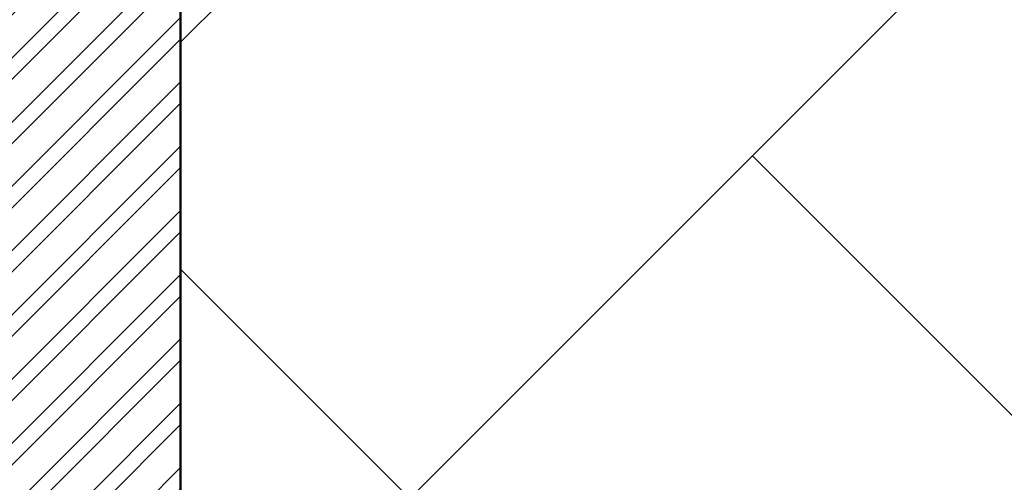
# Model space of a CAD drawing. Units: inches. Extents: x 3590 to 5167, y 65 to 1917.
# Tile 54 of 100: x 4927 to 4968, y 1538 to 1558. Entities that reach past the tile are written whole.
import ezdxf

# ---------------------------------------------------------------- set-up
doc = ezdxf.new("R2010")
doc.units = ezdxf.units.IN
for name, color, linetype, lineweight in [('A-FLOR-PATT', 8, 'Continuous', 13), ('A-WALL', 7, 'Continuous', 50), ('A-WALL-PATT', 251, 'Continuous', 13)]:
    doc.layers.add(name, color=color, linetype=linetype, lineweight=lineweight)

msp = doc.modelspace()

# ---------------------------------------------------------------- hatches: boundary and pattern name
at = {"layer": 'A-FLOR-PATT', "transparency": 33554687}
h = msp.add_hatch(dxfattribs=at)
h.set_pattern_fill('AR-HBONE', color=256, scale=0.2)
h.set_pattern_definition([(45, (-588.972, 0), (0, 28.73682), [60.96, -20.32]), (135, (-574.604, 14.368), (3e-15, 28.73682), [60.96, -20.32])])
h.paths.add_polyline_path([(5071.274, 1796.999), (4933.274, 1796.999), (4933.274, 1753.999), (4962.774, 1753.999, -0.414214), (4928.774, 1719.999), (4933.274, 1718.999), (4933.274, 1334.999), (5071.274, 1334.999)])
h.paths.add_polyline_path([(4951.78, 1521.077), (4951.715, 1521.04), (4951.563, 1520.895)], flags=16)
h.paths.add_polyline_path([(4952.267, 1521.376), (4952.198, 1521.371), (4952.198, 1521.356)], flags=0)
h.paths.add_polyline_path([(4967.051, 1529.728), (4965.231, 1528.694), (4963.411, 1527.714), (4961.756, 1526.851), (4963.589, 1527.449), (4964.036, 1527.478), (4962.975, 1527.249), (4961.76, 1526.852), (4959.792, 1525.834), (4958.005, 1524.895), (4956.24, 1523.93), (4954.504, 1522.919), (4954.129, 1522.682), (4953.361, 1521.997), (4953.366, 1521.998), (4953.605, 1522.064), (4955.106, 1522.761), (4956.921, 1523.434), (4958.678, 1523.915), (4960.358, 1524.2), (4961.945, 1524.286), (4964.171, 1524.108), (4965.958, 1523.309), (4963.863, 1522.976), (4965.187, 1522.499), (4963.366, 1522.497), (4961.545, 1522.487), (4959.764, 1522.461), (4958.304, 1522.419), (4957.974, 1522.388), (4956.307, 1522.232), (4954.718, 1522.071), (4953.251, 1521.899), (4953.525, 1521.623), (4954.331, 1521.379), (4956.243, 1521.23), (4958.039, 1520.93), (4959.684, 1520.483), (4961.16, 1519.896), (4963.107, 1518.8), (4964.393, 1517.325), (4962.973, 1517.726), (4964.558, 1516.661), (4965.407, 1515.708), (4963.507, 1516.322), (4961.68, 1517.005), (4959.935, 1517.745), (4958.282, 1518.528), (4956.732, 1519.343), (4955.295, 1520.175), (4954.672, 1520.572), (4954.513, 1520.627), (4955.658, 1519.318), (4956.703, 1517.982), (4957.644, 1516.647), (4958.485, 1515.334), (4959.55, 1513.524), (4960.438, 1511.769), (4958.841, 1513.62), (4957.452, 1515.325), (4955.819, 1517.459), (4956.665, 1515.448), (4957.111, 1513.923), (4957.447, 1511.714), (4957.076, 1509.793), (4956.538, 1511.11), (4955.992, 1512.569), (4955.444, 1514.125), (4954.898, 1515.735), (4954.357, 1517.356), (4953.824, 1518.943), (4953.305, 1520.452), (4953.065, 1521.116), (4952.971, 1521.146), (4952.949, 1521.086), (4952.73, 1520.199), (4953.37, 1518.024), (4953.757, 1516.373), (4954.051, 1514.765), (4954.264, 1513.221), (4954.471, 1511.131), (4954.497, 1510.402), (4954.409, 1511.76), (4954.264, 1513.221), (4954.051, 1514.765), (4953.757, 1516.373), (4953.37, 1518.024), (4952.877, 1519.698), (4952.716, 1520.141), (4952.533, 1519.059), (4952.374, 1517.789), (4952.219, 1516.312), (4952.046, 1514.6), (4951.833, 1512.626), (4951.557, 1510.363), (4951.203, 1512.168), (4950.852, 1514.339), (4950.985, 1516.376), (4951.66, 1518.286), (4952.593, 1520.481), (4952.357, 1521.13), (4951.855, 1520.328), (4950.839, 1518.908), (4949.777, 1517.587), (4948.916, 1516.617), (4948.111, 1515.256), (4947.089, 1513.554), (4945.889, 1511.615), (4946.326, 1513.402), (4946.562, 1514.249), (4945.528, 1513.327), (4944.581, 1512.531), (4946.018, 1514.508), (4947.204, 1516.048), (4947.893, 1517.313), (4949.307, 1518.764), (4950.414, 1519.767), (4950.451, 1519.806), (4952.267, 1521.376), (4951.645, 1521.493), (4950.404, 1521.18), (4948.044, 1520.359), (4946.119, 1519.452), (4944.572, 1518.475), (4943.35, 1517.443), (4941.997, 1515.92), (4941.661, 1515.275), (4942.813, 1516.99), (4944.572, 1518.475), (4946.119, 1519.452), (4948.044, 1520.359), (4950.404, 1521.18), (4951.645, 1521.493), (4949.647, 1521.868), (4948.6, 1521.756), (4947.126, 1521.57), (4945.42, 1521.348), (4943.45, 1521.105), (4941.183, 1520.856), (4942.86, 1521.613), (4943.873, 1522.03), (4942.952, 1521.909), (4941.41, 1521.485), (4939.543, 1520.67), (4938.968, 1520.226), (4940.733, 1521.299), (4942.952, 1521.909), (4943.702, 1522.008), (4945.894, 1522.7), (4947.565, 1522.714), (4948.921, 1522.566), (4951.131, 1522.183), (4950.971, 1522.297), (4948.129, 1523.006), (4946.035, 1523.707), (4944.232, 1524.521), (4942.707, 1525.461), (4941.444, 1526.537), (4940.43, 1527.761), (4939.649, 1529.143), (4941.421, 1528.122), (4943.147, 1527.132), (4944.841, 1526.175), (4946.514, 1525.25), (4948.179, 1524.359), (4948.365, 1524.263), (4946.475, 1526.045), (4945.181, 1527.54), (4944.19, 1529.033), (4943.496, 1530.54), (4943.278, 1531.36), (4942.498, 1531.919), (4943.114, 1531.762), (4942.959, 1533.659), (4944.14, 1531.989), (4944.612, 1531.323), (4946.202, 1530.463), (4947.486, 1529.509), (4948.79, 1528.226), (4950.368, 1526.237), (4949.485, 1528.155), (4948.851, 1530.123), (4948.491, 1532.041), (4948.381, 1533.918), (4948.501, 1535.76), (4948.827, 1537.573), (4949.418, 1535.565), (4949.957, 1533.569), (4950.464, 1531.586), (4950.961, 1529.617), (4951.391, 1527.954), (4951.724, 1530.687), (4952.201, 1532.58), (4952.889, 1534.33), (4953.77, 1535.951), (4954.827, 1537.46), (4954.521, 1535.39), (4954.273, 1533.937), (4955.58, 1535.663), (4956.748, 1536.739), (4956.159, 1534.78), (4955.589, 1532.873), (4955.043, 1531.006), (4954.525, 1529.166), (4954.038, 1527.341), (4953.638, 1525.733), (4953.611, 1525.586), (4953.398, 1524.166), (4953.382, 1524.009), (4954.07, 1525.476), (4954.912, 1527.022), (4956.136, 1528.894), (4957.847, 1530.577), (4959.376, 1531.54), (4958.256, 1530.104), (4957.143, 1528.663), (4956.066, 1527.243), (4955.056, 1525.871), (4954.141, 1524.571), (4953.352, 1523.372), (4953.311, 1523.303), (4953.273, 1522.925), (4953.261, 1522.382), (4954.103, 1523.373), (4954.63, 1524.284), (4955.961, 1526.358), (4957.23, 1528.13), (4958.421, 1529.609), (4960.037, 1531.368), (4961.374, 1532.375), (4962.101, 1532.77), (4961.07, 1531.061), (4959.987, 1529.438), (4958.869, 1527.908), (4958.15, 1527.007), (4959.803, 1528.003), (4961.589, 1528.793), (4963.391, 1529.328), (4965.211, 1529.632)], flags=16)
h.paths.add_polyline_path([(4962.944, 1523.182), (4961.107, 1523.422), (4960.392, 1523.362), (4962.35, 1523.331)], flags=0)
h.paths.add_polyline_path([(5049.541, 1584.551), (5049.476, 1584.515), (5049.325, 1584.37)], flags=16)
h.paths.add_polyline_path([(5050.028, 1584.851), (5049.959, 1584.845), (5049.959, 1584.83)], flags=0)
h.paths.add_polyline_path([(5042.333, 1581.949), (5043.88, 1582.926), (5045.806, 1583.833), (5048.165, 1584.654), (5049.406, 1584.967), (5047.408, 1585.342), (5046.361, 1585.231), (5044.888, 1585.044), (5043.181, 1584.822), (5041.211, 1584.579), (5038.944, 1584.33), (5040.622, 1585.087), (5041.634, 1585.504), (5040.713, 1585.383), (5039.171, 1584.959), (5037.304, 1584.144), (5036.729, 1583.7), (5038.494, 1584.773), (5040.713, 1585.383), (5041.463, 1585.482), (5043.655, 1586.174), (5045.326, 1586.188), (5046.682, 1586.04), (5048.893, 1585.657), (5048.732, 1585.771), (5045.891, 1586.48), (5043.796, 1587.181), (5041.994, 1587.996), (5040.468, 1588.935), (5039.205, 1590.011), (5038.191, 1591.235), (5037.41, 1592.617), (5039.182, 1591.596), (5040.909, 1590.607), (5042.602, 1589.649), (5044.275, 1588.724), (5045.94, 1587.833), (5046.126, 1587.738), (5044.237, 1589.519), (5042.942, 1591.015), (5041.952, 1592.508), (5041.257, 1594.014), (5041.039, 1594.834), (5040.26, 1595.393), (5040.875, 1595.237), (5040.721, 1597.133), (5041.901, 1595.463), (5042.373, 1594.798), (5043.963, 1593.938), (5045.247, 1592.983), (5046.552, 1591.701), (5048.129, 1589.712), (5047.247, 1591.63), (5046.613, 1593.597), (5046.252, 1595.515), (5046.142, 1597.392), (5046.262, 1599.234), (5046.588, 1601.047), (5047.179, 1599.039), (5047.718, 1597.043), (5048.225, 1595.06), (5048.722, 1593.091), (5049.152, 1591.429), (5049.485, 1594.161), (5049.962, 1596.054), (5050.65, 1597.804), (5051.532, 1599.425), (5052.589, 1600.934), (5052.283, 1598.864), (5052.034, 1597.411), (5053.341, 1599.137), (5054.509, 1600.213), (5053.92, 1598.254), (5053.35, 1596.348), (5052.805, 1594.48), (5052.286, 1592.64), (5051.799, 1590.815), (5051.4, 1589.207), (5051.373, 1589.06), (5051.159, 1587.64), (5051.143, 1587.483), (5051.831, 1588.95), (5052.673, 1590.496), (5053.898, 1592.368), (5055.608, 1594.051), (5057.137, 1595.014), (5056.017, 1593.578), (5054.904, 1592.137), (5053.828, 1590.717), (5052.817, 1589.345), (5051.902, 1588.046), (5051.113, 1586.846), (5051.072, 1586.777), (5051.034, 1586.399), (5051.022, 1585.856), (5051.864, 1586.847), (5052.391, 1587.758), (5053.723, 1589.832), (5054.991, 1591.604), (5056.182, 1593.083), (5057.798, 1594.842), (5059.135, 1595.849), (5059.863, 1596.244), (5058.831, 1594.535), (5057.749, 1592.912), (5056.63, 1591.382), (5055.912, 1590.482), (5057.564, 1591.477), (5059.35, 1592.267), (5061.152, 1592.802), (5062.972, 1593.106), (5064.812, 1593.203), (5062.992, 1592.169), (5061.172, 1591.188), (5059.518, 1590.325), (5061.35, 1590.924), (5061.797, 1590.952), (5060.737, 1590.723), (5059.521, 1590.326), (5057.553, 1589.308), (5055.766, 1588.369), (5054.002, 1587.404), (5052.265, 1586.393), (5051.891, 1586.156), (5051.122, 1585.471), (5051.127, 1585.472), (5051.366, 1585.538), (5052.867, 1586.235), (5054.682, 1586.908), (5056.439, 1587.389), (5058.12, 1587.675), (5059.706, 1587.76), (5061.933, 1587.583), (5063.719, 1586.783), (5061.624, 1586.45), (5062.949, 1585.973), (5061.127, 1585.971), (5059.307, 1585.961), (5057.525, 1585.935), (5056.065, 1585.893), (5055.735, 1585.862), (5054.068, 1585.707), (5052.479, 1585.546), (5051.012, 1585.373), (5051.286, 1585.097), (5052.092, 1584.853), (5054.004, 1584.704), (5055.8, 1584.404), (5057.446, 1583.958), (5058.921, 1583.37), (5060.868, 1582.274), (5062.154, 1580.799), (5060.734, 1581.2), (5062.32, 1580.135), (5063.168, 1579.182), (5061.269, 1579.796), (5059.441, 1580.479), (5057.696, 1581.219), (5056.043, 1582.003), (5054.493, 1582.817), (5053.057, 1583.649), (5052.433, 1584.047), (5052.274, 1584.101), (5053.42, 1582.793), (5054.464, 1581.457), (5055.405, 1580.121), (5056.247, 1578.809), (5057.311, 1576.998), (5058.199, 1575.244), (5056.602, 1577.094), (5055.213, 1578.799), (5053.58, 1580.933), (5054.427, 1578.922), (5054.872, 1577.397), (5055.208, 1575.189), (5054.838, 1573.267), (5054.299, 1574.584), (5053.754, 1576.043), (5053.206, 1577.599), (5052.659, 1579.209), (5052.118, 1580.83), (5051.585, 1582.417), (5051.066, 1583.927), (5050.826, 1584.59), (5050.733, 1584.62), (5050.711, 1584.561), (5050.491, 1583.673), (5051.131, 1581.498), (5051.518, 1579.847), (5051.813, 1578.24), (5052.026, 1576.695), (5052.233, 1574.605), (5052.258, 1573.876), (5052.17, 1575.234), (5052.026, 1576.695), (5051.813, 1578.24), (5051.518, 1579.847), (5051.131, 1581.498), (5050.638, 1583.172), (5050.477, 1583.615), (5050.294, 1582.533), (5050.136, 1581.263), (5049.981, 1579.786), (5049.807, 1578.074), (5049.594, 1576.1), (5049.318, 1573.837), (5048.965, 1575.642), (5048.613, 1577.813), (5048.747, 1579.85), (5049.421, 1581.76), (5050.354, 1583.955), (5050.118, 1584.604), (5049.616, 1583.802), (5048.6, 1582.382), (5047.538, 1581.061), (5046.677, 1580.091), (5045.872, 1578.73), (5044.85, 1577.028), (5043.651, 1575.089), (5044.087, 1576.877), (5044.324, 1577.723), (5043.289, 1576.801), (5042.342, 1576.005), (5043.779, 1577.982), (5044.966, 1579.522), (5045.655, 1580.787), (5047.068, 1582.239), (5048.175, 1583.241), (5048.213, 1583.28), (5050.028, 1584.851), (5049.406, 1584.967), (5048.165, 1584.654), (5045.806, 1583.833), (5043.88, 1582.926), (5042.333, 1581.949), (5041.111, 1580.917), (5039.758, 1579.394), (5039.423, 1578.749), (5040.575, 1580.464)], flags=16)
h.paths.add_polyline_path([(4954.799, 1533.12), (4954.262, 1532.079), (4953.831, 1530.935), (4953.505, 1529.636), (4953.283, 1528.133), (4953.167, 1526.376), (4953.156, 1524.315), (4953.277, 1521.236), (4952.802, 1521.842), (4951.557, 1521.998), (4950.976, 1521.961), (4952.661, 1521.941), (4952.802, 1521.842), (4953.152, 1523.593), (4953.167, 1526.376), (4953.283, 1528.133), (4953.609, 1530.346), (4954.456, 1532.592)], flags=0)
h.paths.add_polyline_path([(5050.563, 1585.316), (5049.318, 1585.472), (5048.737, 1585.435), (5050.422, 1585.415), (5050.563, 1585.316), (5050.914, 1587.067), (5050.928, 1589.851), (5051.045, 1591.607), (5051.371, 1593.82), (5052.217, 1596.066), (5052.56, 1596.594), (5052.024, 1595.554), (5051.592, 1594.409), (5051.266, 1593.11), (5051.045, 1591.607), (5050.928, 1589.851), (5050.918, 1587.789), (5051.038, 1584.71)], flags=0)
h.paths.add_polyline_path([(5058.153, 1586.836), (5060.111, 1586.805), (5060.705, 1586.656), (5058.868, 1586.896)], flags=0)
h.paths.add_polyline_path([(5049.541, 1430.936), (5049.476, 1430.9), (5049.325, 1430.755)], flags=16)
h.paths.add_polyline_path([(5050.028, 1431.236), (5049.959, 1431.231), (5049.959, 1431.215)], flags=0)
h.paths.add_polyline_path([(5046.588, 1447.432), (5047.179, 1445.425), (5047.718, 1443.429), (5048.225, 1441.446), (5048.722, 1439.476), (5049.152, 1437.814), (5049.485, 1440.546), (5049.962, 1442.439), (5050.65, 1444.189), (5051.532, 1445.811), (5052.589, 1447.319), (5052.283, 1445.249), (5052.034, 1443.796), (5053.341, 1445.522), (5054.509, 1446.598), (5053.92, 1444.64), (5053.35, 1442.733), (5052.805, 1440.865), (5052.286, 1439.025), (5051.799, 1437.201), (5051.4, 1435.592), (5051.373, 1435.445), (5051.159, 1434.025), (5051.143, 1433.868), (5051.831, 1435.335), (5052.673, 1436.881), (5053.898, 1438.753), (5055.608, 1440.436), (5057.137, 1441.4), (5056.017, 1439.963), (5054.904, 1438.522), (5053.828, 1437.102), (5052.817, 1435.73), (5051.902, 1434.431), (5051.113, 1433.231), (5051.072, 1433.162), (5051.034, 1432.784), (5051.022, 1432.242), (5051.864, 1433.232), (5052.391, 1434.143), (5053.723, 1436.217), (5054.991, 1437.989), (5056.182, 1439.468), (5057.798, 1441.227), (5059.135, 1442.235), (5059.863, 1442.629), (5058.831, 1440.921), (5057.749, 1439.298), (5056.63, 1437.767), (5055.912, 1436.867), (5057.564, 1437.863), (5059.35, 1438.652), (5061.152, 1439.187), (5062.972, 1439.491), (5064.812, 1439.588), (5062.992, 1438.554), (5061.172, 1437.573), (5059.518, 1436.71), (5061.35, 1437.309), (5061.797, 1437.337), (5060.737, 1437.108), (5059.521, 1436.711), (5057.553, 1435.693), (5055.766, 1434.754), (5054.002, 1433.789), (5052.265, 1432.778), (5051.891, 1432.541), (5051.122, 1431.856), (5051.127, 1431.857), (5051.366, 1431.923), (5052.867, 1432.62), (5054.682, 1433.293), (5056.439, 1433.775), (5058.12, 1434.06), (5059.706, 1434.145), (5061.933, 1433.968), (5063.719, 1433.168), (5061.624, 1432.835), (5062.949, 1432.358), (5061.127, 1432.357), (5059.307, 1432.346), (5057.525, 1432.32), (5056.065, 1432.278), (5055.735, 1432.248), (5054.068, 1432.092), (5052.479, 1431.931), (5051.012, 1431.759), (5051.286, 1431.482), (5052.092, 1431.238), (5054.004, 1431.089), (5055.8, 1430.789), (5057.446, 1430.343), (5058.921, 1429.755), (5060.868, 1428.66), (5062.154, 1427.185), (5060.734, 1427.585), (5062.32, 1426.52), (5063.168, 1425.567), (5061.269, 1426.181), (5059.441, 1426.865), (5057.696, 1427.604), (5056.043, 1428.388), (5054.493, 1429.202), (5053.057, 1430.034), (5052.433, 1430.432), (5052.274, 1430.487), (5053.42, 1429.178), (5054.464, 1427.842), (5055.405, 1426.506), (5056.247, 1425.194), (5057.311, 1423.383), (5058.199, 1421.629), (5056.602, 1423.479), (5055.213, 1425.184), (5053.58, 1427.318), (5054.427, 1425.307), (5054.872, 1423.782), (5055.208, 1421.574), (5054.838, 1419.652), (5054.299, 1420.97), (5053.754, 1422.428), (5053.206, 1423.984), (5052.659, 1425.595), (5052.118, 1427.215), (5051.585, 1428.802), (5051.066, 1430.312), (5050.826, 1430.975), (5050.733, 1431.005), (5050.711, 1430.946), (5050.491, 1430.058), (5051.131, 1427.883), (5051.518, 1426.232), (5051.813, 1424.625), (5052.026, 1423.081), (5052.233, 1420.991), (5052.258, 1420.261), (5052.17, 1421.619), (5052.026, 1423.081), (5051.813, 1424.625), (5051.518, 1426.232), (5051.131, 1427.883), (5050.638, 1429.558), (5050.477, 1430.001), (5050.294, 1428.918), (5050.136, 1427.648), (5049.981, 1426.171), (5049.807, 1424.459), (5049.594, 1422.485), (5049.318, 1420.222), (5048.965, 1422.028), (5048.613, 1424.199), (5048.747, 1426.235), (5049.421, 1428.146), (5050.354, 1430.34), (5050.118, 1430.989), (5049.616, 1430.187), (5048.6, 1428.768), (5047.538, 1427.446), (5046.677, 1426.477), (5045.872, 1425.116), (5044.85, 1423.413), (5043.651, 1421.474), (5044.087, 1423.262), (5044.324, 1424.109), (5043.289, 1423.186), (5042.342, 1422.391), (5043.779, 1424.368), (5044.966, 1425.907), (5045.655, 1427.173), (5047.068, 1428.624), (5048.175, 1429.627), (5048.213, 1429.666), (5050.028, 1431.236), (5049.406, 1431.353), (5048.165, 1431.039), (5045.806, 1430.218), (5043.88, 1429.311), (5042.333, 1428.334), (5041.111, 1427.302), (5039.758, 1425.779), (5039.423, 1425.134), (5040.575, 1426.849), (5042.333, 1428.334), (5043.88, 1429.311), (5045.806, 1430.218), (5048.165, 1431.039), (5049.406, 1431.353), (5047.408, 1431.727), (5046.361, 1431.616), (5044.888, 1431.429), (5043.181, 1431.207), (5041.211, 1430.964), (5038.944, 1430.715), (5040.622, 1431.472), (5041.634, 1431.89), (5040.713, 1431.769), (5039.171, 1431.345), (5037.304, 1430.53), (5036.729, 1430.085), (5038.494, 1431.158), (5040.713, 1431.769), (5041.463, 1431.867), (5043.655, 1432.559), (5045.326, 1432.573), (5046.682, 1432.425), (5048.893, 1432.042), (5048.732, 1432.156), (5045.891, 1432.865), (5043.796, 1433.566), (5041.994, 1434.381), (5040.468, 1435.321), (5039.205, 1436.396), (5038.191, 1437.62), (5037.41, 1439.002), (5039.182, 1437.982), (5040.909, 1436.992), (5042.602, 1436.034), (5044.275, 1435.109), (5045.94, 1434.218), (5046.126, 1434.123), (5044.237, 1435.904), (5042.942, 1437.4), (5041.952, 1438.893), (5041.257, 1440.399), (5041.039, 1441.219), (5040.26, 1441.778), (5040.875, 1441.622), (5040.721, 1443.518), (5041.901, 1441.848), (5042.373, 1441.183), (5043.963, 1440.323), (5045.247, 1439.369), (5046.552, 1438.086), (5048.129, 1436.097), (5047.247, 1438.015), (5046.613, 1439.982), (5046.252, 1441.901), (5046.142, 1443.778), (5046.262, 1445.619)], flags=16)
h.paths.add_polyline_path([(5052.382, 1444.255), (5051.623, 1442.78), (5052.024, 1441.939), (5052.56, 1442.98)], flags=0)
h.paths.add_polyline_path([(5050.563, 1431.701), (5049.318, 1431.857), (5048.737, 1431.821), (5050.422, 1431.8)], flags=0)
h.paths.add_polyline_path([(5058.153, 1433.221), (5060.111, 1433.19), (5060.705, 1433.041), (5058.868, 1433.281)], flags=0)
h.paths.add_polyline_path([(5049.541, 1352.285), (5049.476, 1352.249), (5049.325, 1352.104)], flags=16)
h.paths.add_polyline_path([(5050.028, 1352.585), (5049.959, 1352.58), (5049.959, 1352.564)], flags=0)
h.paths.add_polyline_path([(5046.588, 1368.781), (5047.179, 1366.774), (5047.718, 1364.778), (5048.225, 1362.795), (5048.722, 1360.825), (5049.152, 1359.163), (5049.485, 1361.896), (5049.962, 1363.789), (5050.65, 1365.538), (5051.532, 1367.16), (5052.589, 1368.669), (5052.283, 1366.598), (5052.034, 1365.145), (5053.341, 1366.871), (5054.509, 1367.947), (5053.92, 1365.989), (5053.35, 1364.082), (5052.805, 1362.214), (5052.286, 1360.374), (5051.799, 1358.55), (5051.4, 1356.942), (5051.373, 1356.794), (5051.159, 1355.374), (5051.143, 1355.218), (5051.831, 1356.684), (5052.673, 1358.23), (5053.898, 1360.102), (5055.608, 1361.786), (5057.137, 1362.749), (5056.017, 1361.313), (5054.904, 1359.872), (5053.828, 1358.452), (5052.817, 1357.079), (5051.902, 1355.78), (5051.113, 1354.581), (5051.072, 1354.512), (5051.034, 1354.133), (5051.022, 1353.591), (5051.864, 1354.581), (5052.391, 1355.492), (5053.723, 1357.566), (5054.991, 1359.338), (5056.182, 1360.817), (5057.798, 1362.577), (5059.135, 1363.584), (5059.863, 1363.979), (5058.831, 1362.27), (5057.749, 1360.647), (5056.63, 1359.117), (5055.912, 1358.216), (5057.564, 1359.212), (5059.35, 1360.001), (5061.152, 1360.536), (5062.972, 1360.841), (5064.812, 1360.937), (5062.992, 1359.903), (5061.172, 1358.923), (5059.518, 1358.059), (5061.35, 1358.658), (5061.797, 1358.687), (5060.737, 1358.458), (5059.521, 1358.061), (5057.553, 1357.043), (5055.766, 1356.103), (5054.002, 1355.138), (5052.265, 1354.127), (5051.891, 1353.89), (5051.122, 1353.206), (5051.127, 1353.206), (5051.366, 1353.272), (5052.867, 1353.969), (5054.682, 1354.643), (5056.439, 1355.124), (5058.12, 1355.409), (5059.706, 1355.495), (5061.933, 1355.317), (5063.719, 1354.518), (5061.624, 1354.184), (5062.949, 1353.708), (5061.127, 1353.706), (5059.307, 1353.695), (5057.525, 1353.669), (5056.065, 1353.627), (5055.735, 1353.597), (5054.068, 1353.441), (5052.479, 1353.28), (5051.012, 1353.108), (5051.286, 1352.831), (5052.092, 1352.587), (5054.004, 1352.439), (5055.8, 1352.138), (5057.446, 1351.692), (5058.921, 1351.104), (5060.868, 1350.009), (5062.154, 1348.534), (5060.734, 1348.935), (5062.32, 1347.869), (5063.168, 1346.916), (5061.269, 1347.53), (5059.441, 1348.214), (5057.696, 1348.954), (5056.043, 1349.737), (5054.493, 1350.551), (5053.057, 1351.383), (5052.433, 1351.781), (5052.274, 1351.836), (5053.42, 1350.527), (5054.464, 1349.191), (5055.405, 1347.855), (5056.247, 1346.543), (5057.311, 1344.733), (5058.199, 1342.978), (5056.602, 1344.828), (5055.213, 1346.534), (5053.58, 1348.667), (5054.427, 1346.656), (5054.872, 1345.132), (5055.208, 1342.923), (5054.838, 1341.002), (5054.299, 1342.319), (5053.754, 1343.778), (5053.206, 1345.334), (5052.659, 1346.944), (5052.118, 1348.564), (5051.585, 1350.151), (5051.066, 1351.661), (5050.826, 1352.324), (5050.733, 1352.355), (5050.711, 1352.295), (5050.491, 1351.408), (5051.131, 1349.232), (5051.518, 1347.581), (5051.813, 1345.974), (5052.026, 1344.43), (5052.233, 1342.34), (5052.258, 1341.61), (5052.17, 1342.969), (5052.026, 1344.43), (5051.813, 1345.974), (5051.518, 1347.581), (5051.131, 1349.232), (5050.638, 1350.907), (5050.477, 1351.35), (5050.294, 1350.267), (5050.136, 1348.997), (5049.981, 1347.52), (5049.807, 1345.809), (5049.594, 1343.835), (5049.318, 1341.571), (5048.965, 1343.377), (5048.613, 1345.548), (5048.747, 1347.585), (5049.421, 1349.495), (5050.354, 1351.689), (5050.118, 1352.339), (5049.616, 1351.536), (5048.6, 1350.117), (5047.538, 1348.795), (5046.677, 1347.826), (5045.872, 1346.465), (5044.85, 1344.763), (5043.651, 1342.824), (5044.087, 1344.611), (5044.324, 1345.458), (5043.289, 1344.535), (5042.342, 1343.74), (5043.779, 1345.717), (5044.966, 1347.256), (5045.655, 1348.522), (5047.068, 1349.973), (5048.175, 1350.976), (5048.213, 1351.015), (5050.028, 1352.585), (5049.406, 1352.702), (5048.165, 1352.388), (5045.806, 1351.567), (5043.88, 1350.661), (5042.333, 1349.683), (5041.111, 1348.651), (5039.758, 1347.128), (5039.423, 1346.483), (5040.575, 1348.198), (5042.333, 1349.683), (5043.88, 1350.661), (5045.806, 1351.567), (5048.165, 1352.388), (5049.406, 1352.702), (5047.408, 1353.076), (5046.361, 1352.965), (5044.888, 1352.779), (5043.181, 1352.556), (5041.211, 1352.313), (5038.944, 1352.065), (5040.622, 1352.821), (5041.634, 1353.239), (5040.713, 1353.118), (5039.171, 1352.694), (5037.304, 1351.879), (5036.729, 1351.434), (5038.494, 1352.508), (5040.713, 1353.118), (5041.463, 1353.216), (5043.655, 1353.909), (5045.326, 1353.923), (5046.682, 1353.774), (5048.893, 1353.391), (5048.732, 1353.506), (5045.891, 1354.214), (5043.796, 1354.915), (5041.994, 1355.73), (5040.468, 1356.67), (5039.205, 1357.746), (5038.191, 1358.969), (5037.41, 1360.352), (5039.182, 1359.331), (5040.909, 1358.341), (5042.602, 1357.383), (5044.275, 1356.458), (5045.94, 1355.567), (5046.126, 1355.472), (5044.237, 1357.253), (5042.942, 1358.749), (5041.952, 1360.242), (5041.257, 1361.748), (5041.039, 1362.568), (5040.26, 1363.128), (5040.875, 1362.971), (5040.721, 1364.867), (5041.901, 1363.197), (5042.373, 1362.532), (5043.963, 1361.672), (5045.247, 1360.718), (5046.552, 1359.435), (5048.129, 1357.446), (5047.247, 1359.364), (5046.613, 1361.331), (5046.252, 1363.25), (5046.142, 1365.127), (5046.262, 1366.969)], flags=16)
h.paths.add_polyline_path([(5052.382, 1365.604), (5051.623, 1364.129), (5052.024, 1363.288), (5052.56, 1364.329)], flags=0)
h.paths.add_polyline_path([(4951.78, 1698.041), (4951.715, 1698.005), (4951.563, 1697.859)], flags=16)
h.paths.add_polyline_path([(4952.267, 1698.341), (4952.198, 1698.335), (4952.198, 1698.32)], flags=0)
h.paths.add_polyline_path([(4957.076, 1686.757), (4956.538, 1688.074), (4955.992, 1689.533), (4955.444, 1691.089), (4954.898, 1692.699), (4954.357, 1694.32), (4953.824, 1695.907), (4953.305, 1697.417), (4953.065, 1698.08), (4952.971, 1698.11), (4952.949, 1698.051), (4952.73, 1697.163), (4953.37, 1694.988), (4953.757, 1693.337), (4954.051, 1691.729), (4954.264, 1690.185), (4954.471, 1688.095), (4954.497, 1687.366), (4954.409, 1688.724), (4954.264, 1690.185), (4954.051, 1691.729), (4953.757, 1693.337), (4953.37, 1694.988), (4952.877, 1696.662), (4952.716, 1697.105), (4952.533, 1696.023), (4952.374, 1694.753), (4952.219, 1693.276), (4952.046, 1691.564), (4951.833, 1689.59), (4951.557, 1687.327), (4951.203, 1689.132), (4950.852, 1691.303), (4950.985, 1693.34), (4951.66, 1695.25), (4952.593, 1697.445), (4952.357, 1698.094), (4951.855, 1697.292), (4950.839, 1695.872), (4949.777, 1694.551), (4948.916, 1693.581), (4948.111, 1692.22), (4947.089, 1690.518), (4945.889, 1688.579), (4946.326, 1690.366), (4946.562, 1691.213), (4945.528, 1690.291), (4944.581, 1689.495), (4946.018, 1691.472), (4947.204, 1693.012), (4947.893, 1694.277), (4949.307, 1695.729), (4950.414, 1696.731), (4950.451, 1696.77), (4952.267, 1698.341), (4951.645, 1698.457), (4950.404, 1698.144), (4948.044, 1697.323), (4946.119, 1696.416), (4944.572, 1695.439), (4943.35, 1694.407), (4941.997, 1692.884), (4941.661, 1692.239), (4942.813, 1693.954), (4944.572, 1695.439), (4946.119, 1696.416), (4948.044, 1697.323), (4950.404, 1698.144), (4951.645, 1698.457), (4949.647, 1698.832), (4948.6, 1698.72), (4947.126, 1698.534), (4945.42, 1698.312), (4943.45, 1698.069), (4941.183, 1697.82), (4942.86, 1698.577), (4943.873, 1698.994), (4942.952, 1698.873), (4941.41, 1698.449), (4939.543, 1697.634), (4938.968, 1697.19), (4940.733, 1698.263), (4942.952, 1698.873), (4943.702, 1698.972), (4945.894, 1699.664), (4947.565, 1699.678), (4948.921, 1699.53), (4951.131, 1699.147), (4950.971, 1699.261), (4948.129, 1699.97), (4946.035, 1700.671), (4944.232, 1701.486), (4942.707, 1702.425), (4941.444, 1703.501), (4940.43, 1704.725), (4939.649, 1706.107), (4941.421, 1705.086), (4943.147, 1704.097), (4944.841, 1703.139), (4946.514, 1702.214), (4948.179, 1701.323), (4948.365, 1701.227), (4946.475, 1703.009), (4945.181, 1704.505), (4944.19, 1705.997), (4943.496, 1707.504), (4943.278, 1708.324), (4942.498, 1708.883), (4943.114, 1708.727), (4942.959, 1710.623), (4944.14, 1708.953), (4944.612, 1708.287), (4946.202, 1707.428), (4947.486, 1706.473), (4948.79, 1705.191), (4950.368, 1703.202), (4949.485, 1705.12), (4948.851, 1707.087), (4948.491, 1709.005), (4948.381, 1710.882), (4948.501, 1712.724), (4948.827, 1714.537), (4949.418, 1712.529), (4949.957, 1710.533), (4950.464, 1708.55), (4950.961, 1706.581), (4951.391, 1704.919), (4951.724, 1707.651), (4952.201, 1709.544), (4952.889, 1711.294), (4953.77, 1712.915), (4954.827, 1714.424), (4954.521, 1712.354), (4954.273, 1710.901), (4955.58, 1712.627), (4956.748, 1713.703), (4956.159, 1711.744), (4955.589, 1709.837), (4955.043, 1707.97), (4954.525, 1706.13), (4954.038, 1704.305), (4953.638, 1702.697), (4953.611, 1702.55), (4953.398, 1701.13), (4953.382, 1700.973), (4954.07, 1702.44), (4954.912, 1703.986), (4956.136, 1705.858), (4957.847, 1707.541), (4959.376, 1708.504), (4958.256, 1707.068), (4957.143, 1705.627), (4956.066, 1704.207), (4955.056, 1702.835), (4954.141, 1701.536), (4953.352, 1700.336), (4953.311, 1700.267), (4953.273, 1699.889), (4953.261, 1699.346), (4954.103, 1700.337), (4954.63, 1701.248), (4955.961, 1703.322), (4957.23, 1705.094), (4958.421, 1706.573), (4960.037, 1708.332), (4961.374, 1709.339), (4962.101, 1709.734), (4961.07, 1708.025), (4959.987, 1706.402), (4958.869, 1704.872), (4958.15, 1703.972), (4959.803, 1704.967), (4961.589, 1705.757), (4963.391, 1706.292), (4965.211, 1706.596), (4967.051, 1706.692), (4965.231, 1705.659), (4963.411, 1704.678), (4961.756, 1703.815), (4963.589, 1704.413), (4964.036, 1704.442), (4962.975, 1704.213), (4961.76, 1703.816), (4959.792, 1702.798), (4958.005, 1701.859), (4956.24, 1700.894), (4954.504, 1699.883), (4954.129, 1699.646), (4953.361, 1698.961), (4953.366, 1698.962), (4953.605, 1699.028), (4955.106, 1699.725), (4956.921, 1700.398), (4958.678, 1700.879), (4960.358, 1701.164), (4961.945, 1701.25), (4964.171, 1701.073), (4965.958, 1700.273), (4963.863, 1699.94), (4965.187, 1699.463), (4963.366, 1699.461), (4961.545, 1699.451), (4959.764, 1699.425), (4958.304, 1699.383), (4957.974, 1699.352), (4956.307, 1699.197), (4954.718, 1699.036), (4953.251, 1698.863), (4953.525, 1698.587), (4954.331, 1698.343), (4956.243, 1698.194), (4958.039, 1697.894), (4959.684, 1697.447), (4961.16, 1696.86), (4963.107, 1695.764), (4964.393, 1694.289), (4962.973, 1694.69), (4964.558, 1693.625), (4965.407, 1692.672), (4963.507, 1693.286), (4961.68, 1693.969), (4959.935, 1694.709), (4958.282, 1695.492), (4956.732, 1696.307), (4955.295, 1697.139), (4954.672, 1697.536), (4954.513, 1697.591), (4955.658, 1696.282), (4956.703, 1694.946), (4957.644, 1693.611), (4958.485, 1692.298), (4959.55, 1690.488), (4960.438, 1688.733), (4958.841, 1690.584), (4957.452, 1692.289), (4955.819, 1694.423), (4956.665, 1692.412), (4957.111, 1690.887), (4957.447, 1688.678)], flags=16)
h.paths.add_polyline_path([(5050.563, 1353.05), (5049.318, 1353.207), (5048.737, 1353.17), (5050.422, 1353.15)], flags=0)
h.paths.add_polyline_path([(4951.78, 1351.486), (4951.715, 1351.45), (4951.563, 1351.305)], flags=16)
h.paths.add_polyline_path([(4952.267, 1351.786), (4952.198, 1351.78), (4952.198, 1351.765)], flags=0)
h.paths.add_polyline_path([(4954.827, 1367.869), (4954.521, 1365.799), (4954.273, 1364.346), (4955.58, 1366.072), (4956.748, 1367.148), (4956.159, 1365.19), (4955.589, 1363.283), (4955.043, 1361.415), (4954.525, 1359.575), (4954.038, 1357.751), (4953.638, 1356.142), (4953.611, 1355.995), (4953.398, 1354.575), (4953.382, 1354.418), (4954.07, 1355.885), (4954.912, 1357.431), (4956.136, 1359.303), (4957.847, 1360.986), (4959.376, 1361.95), (4958.256, 1360.513), (4957.143, 1359.072), (4956.066, 1357.652), (4955.056, 1356.28), (4954.141, 1354.981), (4953.352, 1353.781), (4953.311, 1353.712), (4953.273, 1353.334), (4953.261, 1352.792), (4954.103, 1353.782), (4954.63, 1354.693), (4955.961, 1356.767), (4957.23, 1358.539), (4958.421, 1360.018), (4960.037, 1361.777), (4961.374, 1362.785), (4962.101, 1363.179), (4961.07, 1361.471), (4959.987, 1359.848), (4958.869, 1358.317), (4958.15, 1357.417), (4959.803, 1358.413), (4961.589, 1359.202), (4963.391, 1359.737), (4965.211, 1360.041), (4967.051, 1360.138), (4965.231, 1359.104), (4963.411, 1358.123), (4961.756, 1357.26), (4963.589, 1357.859), (4964.036, 1357.887), (4962.975, 1357.658), (4961.76, 1357.261), (4959.792, 1356.243), (4958.005, 1355.304), (4956.24, 1354.339), (4954.504, 1353.328), (4954.129, 1353.091), (4953.361, 1352.406), (4953.366, 1352.407), (4953.605, 1352.473), (4955.106, 1353.17), (4956.921, 1353.843), (4958.678, 1354.325), (4960.358, 1354.61), (4961.945, 1354.695), (4964.171, 1354.518), (4965.958, 1353.718), (4963.863, 1353.385), (4965.187, 1352.908), (4963.366, 1352.907), (4961.545, 1352.896), (4959.764, 1352.87), (4958.304, 1352.828), (4957.974, 1352.798), (4956.307, 1352.642), (4954.718, 1352.481), (4953.251, 1352.309), (4953.525, 1352.032), (4954.331, 1351.788), (4956.243, 1351.639), (4958.039, 1351.339), (4959.684, 1350.893), (4961.16, 1350.305), (4963.107, 1349.21), (4964.393, 1347.735), (4962.973, 1348.135), (4964.558, 1347.07), (4965.407, 1346.117), (4963.507, 1346.731), (4961.68, 1347.414), (4959.935, 1348.154), (4958.282, 1348.938), (4956.732, 1349.752), (4955.295, 1350.584), (4954.672, 1350.982), (4954.513, 1351.036), (4955.658, 1349.728), (4956.703, 1348.392), (4957.644, 1347.056), (4958.485, 1345.744), (4959.55, 1343.933), (4960.438, 1342.179), (4958.841, 1344.029), (4957.452, 1345.734), (4955.819, 1347.868), (4956.665, 1345.857), (4957.111, 1344.332), (4957.447, 1342.124), (4957.076, 1340.202), (4956.538, 1341.52), (4955.992, 1342.978), (4955.444, 1344.534), (4954.898, 1346.145), (4954.357, 1347.765), (4953.824, 1349.352), (4953.305, 1350.862), (4953.065, 1351.525), (4952.971, 1351.555), (4952.949, 1351.496), (4952.73, 1350.608), (4953.37, 1348.433), (4953.757, 1346.782), (4954.051, 1345.175), (4954.264, 1343.631), (4954.471, 1341.541), (4954.497, 1340.811), (4954.409, 1342.169), (4954.264, 1343.631), (4954.051, 1345.175), (4953.757, 1346.782), (4953.37, 1348.433), (4952.877, 1350.108), (4952.716, 1350.551), (4952.533, 1349.468), (4952.374, 1348.198), (4952.219, 1346.721), (4952.046, 1345.009), (4951.833, 1343.035), (4951.557, 1340.772), (4951.203, 1342.578), (4950.852, 1344.749), (4950.985, 1346.785), (4951.66, 1348.696), (4952.593, 1350.89), (4952.357, 1351.539), (4951.855, 1350.737), (4950.839, 1349.318), (4949.777, 1347.996), (4948.916, 1347.027), (4948.111, 1345.665), (4947.089, 1343.963), (4945.889, 1342.024), (4946.326, 1343.812), (4946.562, 1344.659), (4945.528, 1343.736), (4944.581, 1342.941), (4946.018, 1344.918), (4947.204, 1346.457), (4947.893, 1347.723), (4949.307, 1349.174), (4950.414, 1350.177), (4950.451, 1350.216), (4952.267, 1351.786), (4951.645, 1351.903), (4950.404, 1351.589), (4948.044, 1350.768), (4946.119, 1349.861), (4944.572, 1348.884), (4943.35, 1347.852), (4941.997, 1346.329), (4941.661, 1345.684), (4942.813, 1347.399), (4944.572, 1348.884), (4946.119, 1349.861), (4948.044, 1350.768), (4950.404, 1351.589), (4951.645, 1351.903), (4949.647, 1352.277), (4948.6, 1352.166), (4947.126, 1351.979), (4945.42, 1351.757), (4943.45, 1351.514), (4941.183, 1351.265), (4942.86, 1352.022), (4943.873, 1352.44), (4942.952, 1352.319), (4941.41, 1351.895), (4939.543, 1351.08), (4938.968, 1350.635), (4940.733, 1351.708), (4942.952, 1352.319), (4943.702, 1352.417), (4945.894, 1353.109), (4947.565, 1353.123), (4948.921, 1352.975), (4951.131, 1352.592), (4950.971, 1352.706), (4948.129, 1353.415), (4946.035, 1354.116), (4944.232, 1354.931), (4942.707, 1355.871), (4941.444, 1356.946), (4940.43, 1358.17), (4939.649, 1359.552), (4941.421, 1358.532), (4943.147, 1357.542), (4944.841, 1356.584), (4946.514, 1355.659), (4948.179, 1354.768), (4948.365, 1354.673), (4946.475, 1356.454), (4945.181, 1357.95), (4944.19, 1359.443), (4943.496, 1360.949), (4943.278, 1361.769), (4942.498, 1362.328), (4943.114, 1362.172), (4942.959, 1364.068), (4944.14, 1362.398), (4944.612, 1361.733), (4946.202, 1360.873), (4947.486, 1359.919), (4948.79, 1358.636), (4950.368, 1356.647), (4949.485, 1358.565), (4948.851, 1360.532), (4948.491, 1362.451), (4948.381, 1364.328), (4948.501, 1366.169), (4948.827, 1367.982), (4949.418, 1365.975), (4949.957, 1363.979), (4950.464, 1361.995), (4950.961, 1360.026), (4951.391, 1358.364), (4951.724, 1361.096), (4952.201, 1362.989), (4952.889, 1364.739), (4953.77, 1366.361)], flags=16)
h.paths.add_polyline_path([(4954.799, 1363.53), (4954.262, 1362.489), (4953.831, 1361.344), (4953.505, 1360.045), (4953.283, 1358.543), (4953.167, 1356.786), (4953.156, 1354.724), (4953.277, 1351.646), (4952.802, 1352.251), (4951.557, 1352.407), (4950.976, 1352.371), (4952.661, 1352.35), (4952.802, 1352.251), (4953.152, 1354.002), (4953.167, 1356.786), (4953.283, 1358.543), (4953.609, 1360.755), (4954.456, 1363.001)], flags=0)
h.paths.add_polyline_path([(4952.802, 1698.806), (4951.557, 1698.962), (4950.976, 1698.925), (4952.661, 1698.905), (4952.802, 1698.806), (4953.152, 1700.557), (4953.167, 1703.34), (4953.283, 1705.097), (4953.609, 1707.31), (4954.456, 1709.556), (4954.799, 1710.084), (4954.262, 1709.043), (4953.831, 1707.899), (4953.505, 1706.6), (4953.283, 1705.097), (4953.167, 1703.34), (4953.156, 1701.279), (4953.277, 1698.2)], flags=0)
h.paths.add_polyline_path([(4962.944, 1700.146), (4961.107, 1700.386), (4960.392, 1700.326), (4962.35, 1700.295)], flags=0)
h.paths.add_polyline_path([(5058.153, 1354.57), (5060.111, 1354.539), (5060.705, 1354.391), (5058.868, 1354.631)], flags=0)
h.paths.add_polyline_path([(4962.944, 1353.591), (4961.107, 1353.831), (4960.392, 1353.771), (4962.35, 1353.74)], flags=0)
h.paths.add_polyline_path([(5049.541, 1778.72), (5049.476, 1778.684), (5049.325, 1778.539)], flags=16)
h.paths.add_polyline_path([(5050.028, 1779.02), (5049.959, 1779.014), (5049.959, 1778.999)], flags=0)
h.paths.add_polyline_path([(5052.258, 1768.045), (5052.17, 1769.403), (5052.026, 1770.864), (5051.813, 1772.409), (5051.518, 1774.016), (5051.131, 1775.667), (5050.638, 1777.341), (5050.477, 1777.784), (5050.294, 1776.702), (5050.136, 1775.432), (5049.981, 1773.955), (5049.807, 1772.243), (5049.594, 1770.269), (5049.318, 1768.006), (5048.965, 1769.811), (5048.613, 1771.982), (5048.747, 1774.019), (5049.421, 1775.929), (5050.354, 1778.124), (5050.118, 1778.773), (5049.616, 1777.971), (5048.6, 1776.551), (5047.538, 1775.23), (5046.677, 1774.26), (5045.872, 1772.899), (5044.85, 1771.197), (5043.651, 1769.258), (5044.087, 1771.046), (5044.324, 1771.892), (5043.289, 1770.97), (5042.342, 1770.174), (5043.779, 1772.151), (5044.966, 1773.691), (5045.655, 1774.956), (5047.068, 1776.408), (5048.175, 1777.41), (5048.213, 1777.449), (5050.028, 1779.02), (5049.406, 1779.136), (5048.165, 1778.823), (5045.806, 1778.002), (5043.88, 1777.095), (5042.333, 1776.118), (5041.111, 1775.086), (5039.758, 1773.563), (5039.423, 1772.918), (5040.575, 1774.633), (5042.333, 1776.118), (5043.88, 1777.095), (5045.806, 1778.002), (5048.165, 1778.823), (5049.406, 1779.136), (5047.408, 1779.511), (5046.361, 1779.4), (5044.888, 1779.213), (5043.181, 1778.991), (5041.211, 1778.748), (5038.944, 1778.499), (5040.622, 1779.256), (5041.634, 1779.673), (5040.713, 1779.552), (5039.171, 1779.128), (5037.304, 1778.313), (5036.729, 1777.869), (5038.494, 1778.942), (5040.713, 1779.552), (5041.463, 1779.651), (5043.655, 1780.343), (5045.326, 1780.357), (5046.682, 1780.209), (5048.893, 1779.826), (5048.732, 1779.94), (5045.891, 1780.649), (5043.796, 1781.35), (5041.994, 1782.165), (5040.468, 1783.104), (5039.205, 1784.18), (5038.191, 1785.404), (5037.41, 1786.786), (5039.182, 1785.765), (5040.909, 1784.776), (5042.602, 1783.818), (5044.275, 1782.893), (5045.94, 1782.002), (5046.126, 1781.907), (5044.237, 1783.688), (5042.942, 1785.184), (5041.952, 1786.677), (5041.257, 1788.183), (5041.039, 1789.003), (5040.26, 1789.562), (5040.875, 1789.406), (5040.721, 1791.302), (5041.901, 1789.632), (5042.373, 1788.967), (5043.963, 1788.107), (5045.247, 1787.152), (5046.552, 1785.87), (5048.129, 1783.881), (5047.247, 1785.799), (5046.613, 1787.766), (5046.252, 1789.684), (5046.142, 1791.561), (5046.262, 1793.403), (5046.588, 1795.216), (5047.179, 1793.208), (5047.718, 1791.213), (5048.225, 1789.229), (5048.722, 1787.26), (5049.152, 1785.598), (5049.485, 1788.33), (5049.962, 1790.223), (5050.65, 1791.973), (5051.532, 1793.594), (5052.589, 1795.103), (5052.283, 1793.033), (5052.034, 1791.58), (5053.341, 1793.306), (5054.509, 1794.382), (5053.92, 1792.423), (5053.35, 1790.517), (5052.805, 1788.649), (5052.286, 1786.809), (5051.799, 1784.984), (5051.4, 1783.376), (5051.373, 1783.229), (5051.159, 1781.809), (5051.143, 1781.652), (5051.831, 1783.119), (5052.673, 1784.665), (5053.898, 1786.537), (5055.608, 1788.22), (5057.137, 1789.183), (5056.017, 1787.747), (5054.904, 1786.306), (5053.828, 1784.886), (5052.817, 1783.514), (5051.902, 1782.215), (5051.113, 1781.015), (5051.072, 1780.946), (5051.034, 1780.568), (5051.022, 1780.025), (5051.864, 1781.016), (5052.391, 1781.927), (5053.723, 1784.001), (5054.991, 1785.773), (5056.182, 1787.252), (5057.798, 1789.011), (5059.135, 1790.018), (5059.863, 1790.413), (5058.831, 1788.704), (5057.749, 1787.081), (5056.63, 1785.551), (5055.912, 1784.651), (5057.564, 1785.646), (5059.35, 1786.436), (5061.152, 1786.971), (5062.972, 1787.275), (5064.812, 1787.372), (5062.992, 1786.338), (5061.172, 1785.357), (5059.518, 1784.494), (5061.35, 1785.093), (5061.797, 1785.121), (5060.737, 1784.892), (5059.521, 1784.495), (5057.553, 1783.477), (5055.766, 1782.538), (5054.002, 1781.573), (5052.265, 1780.562), (5051.891, 1780.325), (5051.122, 1779.64), (5051.127, 1779.641), (5051.366, 1779.707), (5052.867, 1780.404), (5054.682, 1781.077), (5056.439, 1781.558), (5058.12, 1781.844), (5059.706, 1781.929), (5061.933, 1781.752), (5063.719, 1780.952), (5061.624, 1780.619), (5062.949, 1780.142), (5061.127, 1780.14), (5059.307, 1780.13), (5057.525, 1780.104), (5056.065, 1780.062), (5055.735, 1780.031), (5054.068, 1779.876), (5052.479, 1779.715), (5051.012, 1779.542), (5051.286, 1779.266), (5052.092, 1779.022), (5054.004, 1778.873), (5055.8, 1778.573), (5057.446, 1778.127), (5058.921, 1777.539), (5060.868, 1776.443), (5062.154, 1774.968), (5060.734, 1775.369), (5062.32, 1774.304), (5063.168, 1773.351), (5061.269, 1773.965), (5059.441, 1774.648), (5057.696, 1775.388), (5056.043, 1776.172), (5054.493, 1776.986), (5053.057, 1777.818), (5052.433, 1778.216), (5052.274, 1778.27), (5053.42, 1776.962), (5054.464, 1775.626), (5055.405, 1774.29), (5056.247, 1772.978), (5057.311, 1771.167), (5058.199, 1769.413), (5056.602, 1771.263), (5055.213, 1772.968), (5053.58, 1775.102), (5054.427, 1773.091), (5054.872, 1771.566), (5055.208, 1769.358), (5054.838, 1767.436), (5054.299, 1768.753), (5053.754, 1770.212), (5053.206, 1771.768), (5052.659, 1773.378), (5052.118, 1774.999), (5051.585, 1776.586), (5051.066, 1778.096), (5050.826, 1778.759), (5050.733, 1778.789), (5050.711, 1778.73), (5050.491, 1777.842), (5051.131, 1775.667), (5051.518, 1774.016), (5051.813, 1772.409), (5052.026, 1770.864), (5052.233, 1768.774)], flags=16)
h.paths.add_polyline_path([(5050.563, 1779.485), (5049.318, 1779.641), (5048.737, 1779.604), (5050.422, 1779.584), (5050.563, 1779.485), (5050.914, 1781.236), (5050.928, 1784.02), (5051.045, 1785.776), (5051.371, 1787.989), (5052.217, 1790.235), (5052.56, 1790.763), (5052.024, 1789.723), (5051.592, 1788.578), (5051.266, 1787.279), (5051.045, 1785.776), (5050.928, 1784.02), (5050.918, 1781.958), (5051.038, 1778.879)], flags=0)
h.paths.add_polyline_path([(5058.153, 1781.005), (5060.111, 1780.974), (5060.705, 1780.825), (5058.868, 1781.065)], flags=0)
at = {"layer": 'A-WALL-PATT', "transparency": 33554687}
h = msp.add_hatch(dxfattribs=at)
h.set_pattern_fill('ANSI32', color=256, scale=0.2)
h.paths.add_polyline_path([(4684.274, 1805.999), (4591.274, 1805.999), (4591.274, 1796.999), (4639.274, 1796.999), (4639.274, 1790.999), (4648.274, 1790.999), (4648.274, 1796.999), (4684.274, 1796.999)])
h.paths.add_polyline_path([(4543.274, 1805.999), (4420.274, 1805.999), (4420.274, 1784.999), (4429.274, 1784.999), (4429.274, 1796.999), (4445.919, 1796.999), (4543.274, 1796.999)])
h.paths.add_polyline_path([(4828.274, 1805.999), (4744.274, 1805.999), (4744.274, 1796.999), (4828.274, 1796.999)])
h.paths.add_polyline_path([(4648.274, 1754.999), (4639.274, 1754.999), (4639.274, 1655.999), (4546.274, 1655.999), (4546.274, 1649.999), (4549.274, 1649.999), (4549.274, 1553.999), (4429.274, 1553.999), (4429.274, 1583.999), (4420.274, 1583.999), (4420.274, 1538.999), (4429.274, 1538.999), (4429.274, 1544.999), (4639.274, 1544.999), (4639.274, 1538.999), (4648.274, 1538.999), (4648.274, 1559.999), (4639.274, 1559.999), (4639.274, 1553.999), (4555.274, 1553.999), (4555.274, 1649.999), (4639.274, 1649.999), (4639.274, 1589.999), (4648.274, 1589.999)])
h.paths.add_polyline_path([(4516.274, 1655.999), (4429.274, 1655.999), (4429.274, 1736.999), (4420.274, 1736.999), (4420.274, 1619.999), (4429.274, 1619.999), (4429.274, 1649.999), (4516.274, 1649.999)], flags=17)
h.paths.add_polyline_path([(5080.274, 1805.999), (4888.274, 1805.999), (4888.274, 1796.999), (4924.274, 1796.999), (4924.274, 1754.999), (4933.274, 1754.999), (4933.274, 1796.999), (5071.274, 1796.999), (5071.274, 1334.999), (4933.274, 1334.999), (4933.274, 1565.999), (4924.274, 1565.999), (4924.274, 1334.999), (4898.774, 1334.999), (4898.774, 1325.999), (5080.274, 1325.999)])
h.paths.add_polyline_path([(4933.274, 1718.999), (4924.274, 1718.999), (4924.274, 1637.999), (4933.274, 1637.999)], flags=17)
h.paths.add_polyline_path([(4802.774, 1334.999), (4777.274, 1334.999), (4777.274, 1502.999), (4756.274, 1502.999), (4756.274, 1493.999), (4768.274, 1493.999), (4768.274, 1430.999), (4696.274, 1430.999), (4696.274, 1493.999), (4708.274, 1493.999), (4708.274, 1502.999), (4639.274, 1502.999), (4639.274, 1493.999), (4687.274, 1493.999), (4687.274, 1430.999), (4681.274, 1430.999), (4681.274, 1421.999), (4768.274, 1421.999), (4768.274, 1334.999), (4726.274, 1334.999), (4726.274, 1325.999), (4802.774, 1325.999)])
h.paths.add_polyline_path([(4690.274, 1334.999), (4648.274, 1334.999), (4648.274, 1352.867), (4648.274, 1421.999), (4651.274, 1421.999), (4651.274, 1430.999), (4639.274, 1430.999), (4639.274, 1334.999), (4633.274, 1334.999), (4633.274, 1325.999), (4690.274, 1325.999)])
h.paths.add_polyline_path([(4585.274, 1334.999), (4584.724, 1334.999), (4429.274, 1334.999), (4429.274, 1490.999), (4420.274, 1490.999), (4420.274, 1325.999), (4585.274, 1325.999)])

# ---------------------------------------------------------------- linework, layer by layer
at = {"layer": 'A-WALL'}
msp.add_line((4933.274, 1334.999), (4933.274, 1718.999), dxfattribs=at)

doc.saveas('drawing.dxf')
